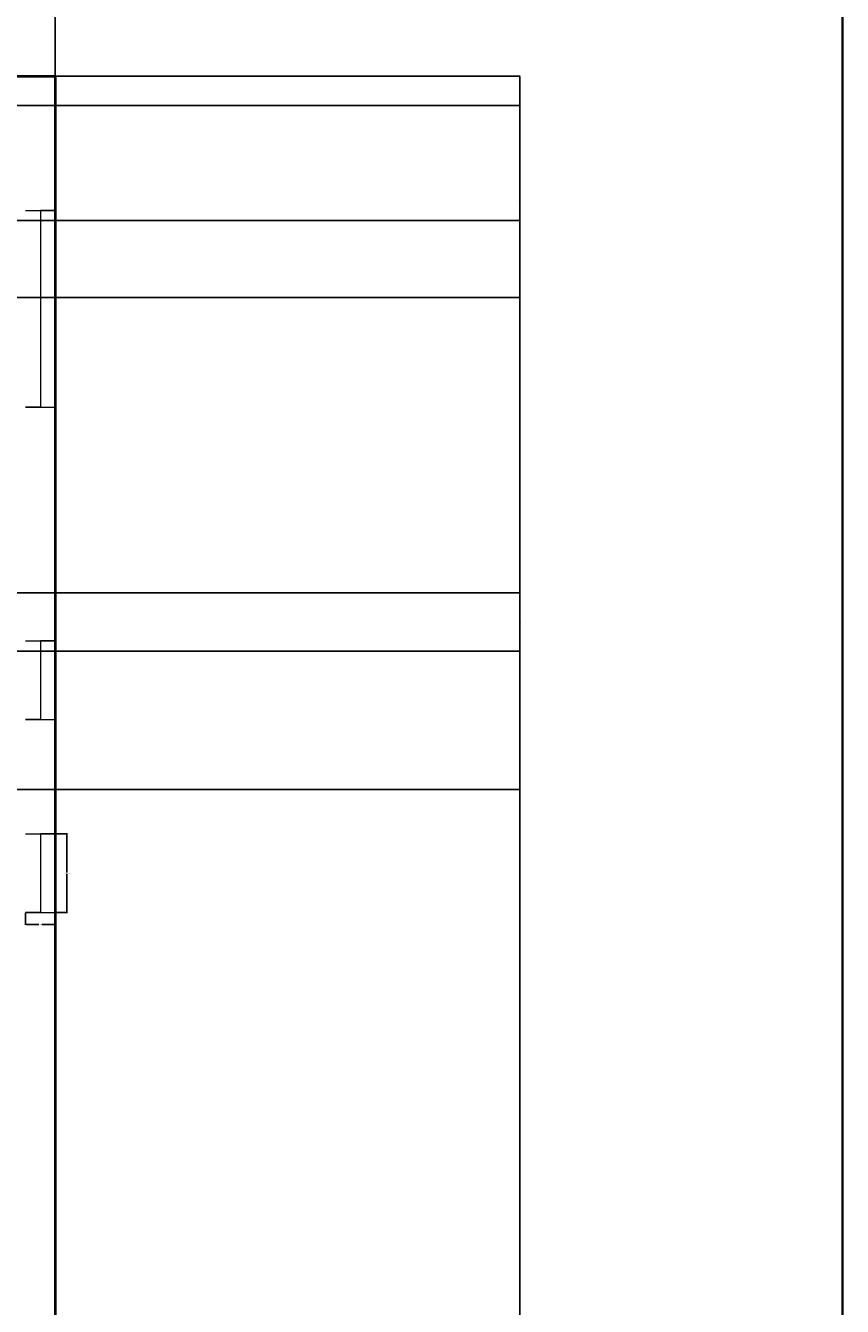
# Model space of a CAD drawing. Units: inches. Extents: x 1355 to 2746, y 1171 to 2751.
# Tile 18 of 24: x 2497 to 2746, y 1764 to 2155. Entities that reach past the tile are written whole.
import ezdxf

# ---------------------------------------------------------------- set-up
doc = ezdxf.new("R2010")
doc.units = ezdxf.units.IN
for name, color, linetype, lineweight in [('A-ANNO-DIMS', 2, 'Continuous', 18), ('A-ANNO-TTLB', 7, 'Continuous', 35), ('A-GLAZ', 4, 'Continuous', 18), ('A-WALL', 7, 'Continuous', 40)]:
    doc.layers.add(name, color=color, linetype=linetype, lineweight=lineweight)
doc.styles.get("Standard").update_dxf_attribs({"font": 'arial.ttf'})
doc.dimstyles.get("Standard").update_dxf_attribs({"dimtxt": 0.18, "dimasz": 0.18, "dimexe": 0.18, "dimexo": 0.0625, "dimgap": 0.09, "dimtad": 0, "dimtih": 1, "dimtoh": 1, "dimdec": 4, "dimzin": 0, "dimdsep": 46, "dimtxsty": 'Standard', "dimcen": 0.09, "dimadec": 0, "dimazin": 0, "dimtfac": 1, "dimtdec": 4, "dimtofl": 0, "dimtmove": 0, "dimatfit": 3, "dimfxl": 1, "dimtolj": 1, "dimtzin": 0, "dimarcsym": 0})

# ---------------------------------------------------------------- blocks, each defined once
blk = doc.blocks.new('WINDOW-PLAN-24')
for p, q in [((0, 24), (9, 24)), ((9, 24), (4.5, 24)), ((4.5, 24), (4.5, 0)), ((4.5, 0), (0, 0)), ((0, 0), (9, 0))]:
    blk.add_line(p, q)
blk = doc.blocks.new('WINDOW-PLAN-24-2')
for p, q in [((0, 24), (9, 24)), ((9, 24), (4.5, 24)), ((4.5, 24), (4.5, 0)), ((4.5, 0), (0, 0)), ((0, 0), (0, 0)), ((0, 0), (9, 0))]:
    blk.add_line(p, q)
blk = doc.blocks.new('WINDOW-PLAN-60')
for p, q in [((0, 60), (9, 60)), ((9, 60), (4.5, 60)), ((4.5, 60), (4.5, 0)), ((4.5, 0), (0, 0)), ((0, 0), (9, 0))]:
    blk.add_line(p, q)
blk = doc.blocks.new('*D49')
at = {"layer": 'A-ANNO-DIMS', "color": 0, "lineweight": -2, "transparency": 16777216}
for p, q in [((2506.45, 1908.33), (2510.17, 1908.33)), ((2509.99, 1908.15), (2509.99, 1896.52)), ((2509.99, 1884.51), (2509.99, 1896.15)), ((2506.45, 1884.33), (2510.17, 1884.33))]:
    blk.add_line(p, q, dxfattribs=at)
at = {"layer": 'A-ANNO-DIMS', "color": 0, "transparency": 16777216}
for points in [[(2509.96, 1908.15), (2510.02, 1908.15), (2509.99, 1908.33)], [(2509.96, 1884.51), (2510.02, 1884.51), (2509.99, 1884.33)]]:
    blk.add_solid(points, dxfattribs=at)
at = {"layer": 'Defpoints', "color": 0, "transparency": 16777216}
for p in [(2506.39, 1908.33), (2509.99, 1908.33), (2506.39, 1884.33)]:
    blk.add_point(p, dxfattribs=at)
at = {"layer": 'A-ANNO-DIMS', "color": 0, "transparency": 16777216, "insert": (2509.99, 1896.33), "char_height": 0.18, "attachment_point": 5}
blk.add_mtext('\\A1;WINDOW 24 TYP.', dxfattribs=at)
blk = doc.blocks.new('*D50')
at = {"layer": 'A-ANNO-DIMS', "color": 0, "lineweight": -2, "transparency": 16777216}
for p, q in [((2497.39, 1884.27), (2497.39, 1880.55)), ((2506.39, 1884.27), (2506.39, 1880.55)), ((2497.57, 1880.73), (2501.43, 1880.73)), ((2506.21, 1880.73), (2502.35, 1880.73))]:
    blk.add_line(p, q, dxfattribs=at)
at = {"layer": 'A-ANNO-DIMS', "color": 0, "transparency": 16777216}
for points in [[(2497.57, 1880.76), (2497.57, 1880.7), (2497.39, 1880.73)], [(2506.21, 1880.76), (2506.21, 1880.7), (2506.39, 1880.73)]]:
    blk.add_solid(points, dxfattribs=at)
at = {"layer": 'Defpoints', "color": 0, "transparency": 16777216}
for p in [(2497.39, 1884.33), (2506.39, 1884.33), (2506.39, 1880.73)]:
    blk.add_point(p, dxfattribs=at)
at = {"layer": 'A-ANNO-DIMS', "color": 0, "transparency": 16777216, "insert": (2501.89, 1880.73), "char_height": 0.18, "attachment_point": 5}
blk.add_mtext('\\A1;9 TYP.', dxfattribs=at)
blk = doc.blocks.new('*D98')
at = {"layer": 'A-ANNO-DIMS', "color": 0, "lineweight": -2, "transparency": 16777216}
for p, q in [((2506.45, 2139.3), (2648.07, 2139.3)), ((2647.89, 2139.12), (2647.89, 1725.48)), ((2647.89, 1311.48), (2647.89, 1725.12)), ((2506.45, 1311.3), (2648.07, 1311.3))]:
    blk.add_line(p, q, dxfattribs=at)
at = {"layer": 'A-ANNO-DIMS', "color": 0, "transparency": 16777216}
for points in [[(2647.86, 2139.12), (2647.92, 2139.12), (2647.89, 2139.3)], [(2647.86, 1311.48), (2647.92, 1311.48), (2647.89, 1311.3)]]:
    blk.add_solid(points, dxfattribs=at)
at = {"layer": 'Defpoints', "color": 0, "transparency": 16777216}
for p in [(2506.39, 2139.3), (2647.89, 2139.3), (2506.39, 1311.3)]:
    blk.add_point(p, dxfattribs=at)
at = {"layer": 'A-ANNO-DIMS', "color": 0, "transparency": 16777216, "insert": (2647.89, 1725.3), "char_height": 0.18, "attachment_point": 5}
blk.add_mtext('\\A1;828', dxfattribs=at)
blk = doc.blocks.new('*D101')
at = {"layer": 'A-ANNO-DIMS', "color": 0, "lineweight": -2, "transparency": 16777216}
for p, q in [((2360.89, 2139.36), (2360.89, 2716.58)), ((2361.07, 2716.4), (2433.25, 2716.4)), ((2506.21, 2716.4), (2434.03, 2716.4)), ((2506.39, 2139.36), (2506.39, 2716.58))]:
    blk.add_line(p, q, dxfattribs=at)
at = {"layer": 'A-ANNO-DIMS', "color": 0, "transparency": 16777216}
for points in [[(2361.07, 2716.43), (2361.07, 2716.37), (2360.89, 2716.4)], [(2506.21, 2716.43), (2506.21, 2716.37), (2506.39, 2716.4)]]:
    blk.add_solid(points, dxfattribs=at)
at = {"layer": 'Defpoints', "color": 0, "transparency": 16777216}
for p in [(2506.39, 2716.4), (2360.89, 2139.3), (2506.39, 2139.3)]:
    blk.add_point(p, dxfattribs=at)
at = {"layer": 'A-ANNO-DIMS', "color": 0, "transparency": 16777216, "insert": (2433.64, 2716.4), "char_height": 0.18, "attachment_point": 5}
blk.add_mtext('\\A1;145.5', dxfattribs=at)
blk = doc.blocks.new('*D110')
at = {"layer": 'A-ANNO-DIMS', "color": 0, "lineweight": -2, "transparency": 16777216}
for p, q in [((2089.45, 2130.3), (2648.07, 2130.3)), ((2647.89, 2130.12), (2647.89, 2101.25)), ((2647.89, 2072.02), (2647.89, 2100.89)), ((2089.45, 2071.84), (2648.07, 2071.84))]:
    blk.add_line(p, q, dxfattribs=at)
at = {"layer": 'A-ANNO-DIMS', "color": 0, "transparency": 16777216}
for points in [[(2647.86, 2130.12), (2647.92, 2130.12), (2647.89, 2130.3)], [(2647.86, 2072.02), (2647.92, 2072.02), (2647.89, 2071.84)]]:
    blk.add_solid(points, dxfattribs=at)
at = {"layer": 'Defpoints', "color": 0, "transparency": 16777216}
for p in [(2089.39, 2130.3), (2647.89, 2130.3), (2089.39, 2071.84)]:
    blk.add_point(p, dxfattribs=at)
at = {"layer": 'A-ANNO-DIMS', "color": 0, "transparency": 16777216, "insert": (2647.89, 2101.07), "char_height": 0.18, "attachment_point": 5}
blk.add_mtext('\\A1;58.46', dxfattribs=at)
blk = doc.blocks.new('*D113')
at = {"layer": 'A-ANNO-DIMS', "color": 0, "lineweight": -2, "transparency": 16777216}
for p, q in [((2225.95, 2139.3), (2648.07, 2139.3)), ((2647.89, 2139.12), (2647.89, 2117.44)), ((2647.89, 2095.4), (2647.89, 2117.08)), ((2225.95, 2095.22), (2648.07, 2095.22))]:
    blk.add_line(p, q, dxfattribs=at)
at = {"layer": 'A-ANNO-DIMS', "color": 0, "transparency": 16777216}
for points in [[(2647.86, 2139.12), (2647.92, 2139.12), (2647.89, 2139.3)], [(2647.86, 2095.4), (2647.92, 2095.4), (2647.89, 2095.22)]]:
    blk.add_solid(points, dxfattribs=at)
at = {"layer": 'Defpoints', "color": 0, "transparency": 16777216}
for p in [(2225.89, 2139.3), (2647.89, 2139.3), (2225.89, 2095.22)]:
    blk.add_point(p, dxfattribs=at)
at = {"layer": 'A-ANNO-DIMS', "color": 0, "transparency": 16777216, "insert": (2647.89, 2117.26), "char_height": 0.18, "attachment_point": 5}
blk.add_mtext('\\A1;44.08', dxfattribs=at)
blk = doc.blocks.new('*D126')
at = {"layer": 'A-ANNO-DIMS', "color": 0, "lineweight": -2, "transparency": 16777216}
for p, q in [((2080.39, 2219.34), (2080.39, 1171.06)), ((2506.39, 2219.34), (2506.39, 1171.06)), ((2080.57, 1171.24), (2293.1, 1171.24)), ((2506.21, 1171.24), (2293.68, 1171.24))]:
    blk.add_line(p, q, dxfattribs=at)
at = {"layer": 'A-ANNO-DIMS', "color": 0, "transparency": 16777216}
for points in [[(2080.57, 1171.27), (2080.57, 1171.21), (2080.39, 1171.24)], [(2506.21, 1171.27), (2506.21, 1171.21), (2506.39, 1171.24)]]:
    blk.add_solid(points, dxfattribs=at)
at = {"layer": 'Defpoints', "color": 0, "transparency": 16777216}
for p in [(2080.39, 2219.4), (2506.39, 2219.4), (2506.39, 1171.24)]:
    blk.add_point(p, dxfattribs=at)
at = {"layer": 'A-ANNO-DIMS', "color": 0, "transparency": 16777216, "insert": (2293.39, 1171.24), "char_height": 0.18, "attachment_point": 5}
blk.add_mtext('\\A1;426', dxfattribs=at)
blk = doc.blocks.new('*D136')
at = {"layer": 'A-ANNO-DIMS', "color": 0, "lineweight": -2, "transparency": 16777216}
for p, q in [((1618.27, 1981.8), (2648.07, 1981.8)), ((2647.89, 1981.62), (2647.89, 1951.98)), ((2647.89, 1921.98), (2647.89, 1951.62)), ((1618.27, 1921.8), (2648.07, 1921.8))]:
    blk.add_line(p, q, dxfattribs=at)
at = {"layer": 'A-ANNO-DIMS', "color": 0, "transparency": 16777216}
for points in [[(2647.86, 1981.62), (2647.92, 1981.62), (2647.89, 1981.8)], [(2647.86, 1921.98), (2647.92, 1921.98), (2647.89, 1921.8)]]:
    blk.add_solid(points, dxfattribs=at)
at = {"layer": 'Defpoints', "color": 0, "transparency": 16777216}
for p in [(1618.21, 1981.8), (2647.89, 1981.8), (1618.21, 1921.8)]:
    blk.add_point(p, dxfattribs=at)
at = {"layer": 'A-ANNO-DIMS', "color": 0, "transparency": 16777216, "insert": (2647.89, 1951.8), "char_height": 0.18, "attachment_point": 5}
blk.add_mtext('\\A1;60', dxfattribs=at)
blk = doc.blocks.new('*D139')
at = {"layer": 'A-ANNO-DIMS', "color": 0, "lineweight": -2, "transparency": 16777216}
for p, q in [((1523.77, 1981.8), (2648.07, 1981.8)), ((2647.89, 1981.62), (2647.89, 1973.09)), ((2647.89, 1964.19), (2647.89, 1972.72)), ((1548.66, 1964.01), (2648.07, 1964.01))]:
    blk.add_line(p, q, dxfattribs=at)
at = {"layer": 'A-ANNO-DIMS', "color": 0, "transparency": 16777216}
for points in [[(2647.86, 1981.62), (2647.92, 1981.62), (2647.89, 1981.8)], [(2647.86, 1964.19), (2647.92, 1964.19), (2647.89, 1964.01)]]:
    blk.add_solid(points, dxfattribs=at)
at = {"layer": 'Defpoints', "color": 0, "transparency": 16777216}
for p in [(1523.71, 1981.8), (1548.6, 1964.01), (2647.89, 1964.01)]:
    blk.add_point(p, dxfattribs=at)
at = {"layer": 'A-ANNO-DIMS', "color": 0, "transparency": 16777216, "insert": (2647.89, 1972.9), "char_height": 0.18, "attachment_point": 5}
blk.add_mtext('\\A1;17.795', dxfattribs=at)

msp = doc.modelspace()

# ---------------------------------------------------------------- linework, layer by layer
at = {"layer": 'A-ANNO-TTLB'}
msp.add_lwpolyline([(1355.0901, 2751.4741), (2746.1804, 2751.4741), (2746.1804, 1182.883), (1355.0901, 1182.883)], close=True, dxfattribs=at)
at = {"layer": 'A-WALL'}
for p, q in [((2360.8909, 2139.3018), (2506.3909, 2139.3018)), ((2506.3909, 2139.3018), (2506.3909, 1311.3018))]:
    msp.add_line(p, q, dxfattribs=at)

# ---------------------------------------------------------------- block references
at = {"layer": 'A-GLAZ'}
for name, p in [('WINDOW-PLAN-60', (2497.3906, 2038.333)), ('WINDOW-PLAN-24', (2497.3906, 1943.194)), ('WINDOW-PLAN-24-2', (2497.3906, 1884.332))]:
    msp.add_blockref(name, p, dxfattribs=at)

# ---------------------------------------------------------------- dimensions: what is measured, and where the dimension line sits
at = {"layer": 'A-ANNO-DIMS'}
for base, p1, p2, override, picture, middle in [((2506.3909, 2716.3999), (2360.8909, 2139.3018), (2506.3909, 2139.3018), {"dimdec": 1, "dimlfac": 1, "dimrnd": 0, "dimzin": 0, "dimdsep": 46, "dimlunit": 2}, '*D101', (2433.6409, 2716.3999)), ((2506.3909, 1171.2388), (2080.3909, 2219.3999), (2506.3909, 2219.3999), {"dimdec": 0, "dimlfac": 1, "dimrnd": 0, "dimzin": 0, "dimdsep": 46, "dimlunit": 2}, '*D126', (2293.3909, 1171.2388))]:
    dim = msp.add_linear_dim(base=base, p1=p1, p2=p2, dimstyle='Standard', override=override, dxfattribs=at)
    dim.commit()
    dim.dimension.update_dxf_attribs({"geometry": picture, "text_midpoint": middle})
for base, p1, p2, override, picture, middle in [((2647.886, 2139.3018), (2225.8909, 2095.2225), (2225.8909, 2139.3018), {"dimdec": 2, "dimlfac": 1, "dimrnd": 0, "dimzin": 0, "dimdsep": 46, "dimlunit": 2}, '*D113', (2647.886, 2117.2622)), ((2647.886, 2139.3018), (2506.3909, 1311.3018), (2506.3909, 2139.3018), {"dimdec": 0, "dimlfac": 1, "dimrnd": 0, "dimzin": 0, "dimdsep": 46, "dimlunit": 2}, '*D98', (2647.886, 1725.3018)), ((2647.886, 2130.3018), (2089.3909, 2071.8385), (2089.3909, 2130.3018), {"dimdec": 2, "dimlfac": 1, "dimrnd": 0, "dimzin": 0, "dimdsep": 46, "dimlunit": 2}, '*D110', (2647.886, 2101.0702)), ((2647.886, 1964.0069), (1523.7083, 1981.8018), (1548.5973, 1964.0069), {"dimdec": 3, "dimlfac": 1, "dimrnd": 0, "dimzin": 0, "dimdsep": 46, "dimlunit": 2}, '*D139', (2647.886, 1972.9044)), ((2647.886, 1981.8018), (1618.2083, 1921.8018), (1618.2083, 1981.8018), {"dimdec": 0, "dimlfac": 1, "dimrnd": 0, "dimzin": 0, "dimdsep": 46, "dimlunit": 2}, '*D136', (2647.886, 1951.8018))]:
    dim = msp.add_linear_dim(base=base, p1=p1, p2=p2, angle=90, dimstyle='Standard', override=override, dxfattribs=at)
    dim.commit()
    dim.dimension.update_dxf_attribs({"geometry": picture, "text_midpoint": middle})
dim = msp.add_linear_dim(base=(2509.9909, 1908.3321), p1=(2506.3909, 1884.3321), p2=(2506.3909, 1908.3321), angle=90, text='WINDOW <> TYP.', dimstyle='Standard', override={"dimdec": 0, "dimlfac": 1, "dimrnd": 0, "dimzin": 0, "dimdsep": 46, "dimlunit": 2}, dxfattribs=at)
dim.commit()
dim.dimension.update_dxf_attribs({"geometry": '*D49', "text_midpoint": (2509.9909, 1896.3321)})
dim = msp.add_linear_dim(base=(2506.3909, 1880.7321), p1=(2497.3909, 1884.3321), p2=(2506.3909, 1884.3321), text='<> TYP.', dimstyle='Standard', override={"dimdec": 0, "dimlfac": 1, "dimrnd": 0, "dimzin": 0, "dimdsep": 46, "dimlunit": 2}, dxfattribs=at)
dim.commit()
dim.dimension.update_dxf_attribs({"geometry": '*D50', "text_midpoint": (2501.8909, 1880.7321)})

doc.saveas('drawing.dxf')
